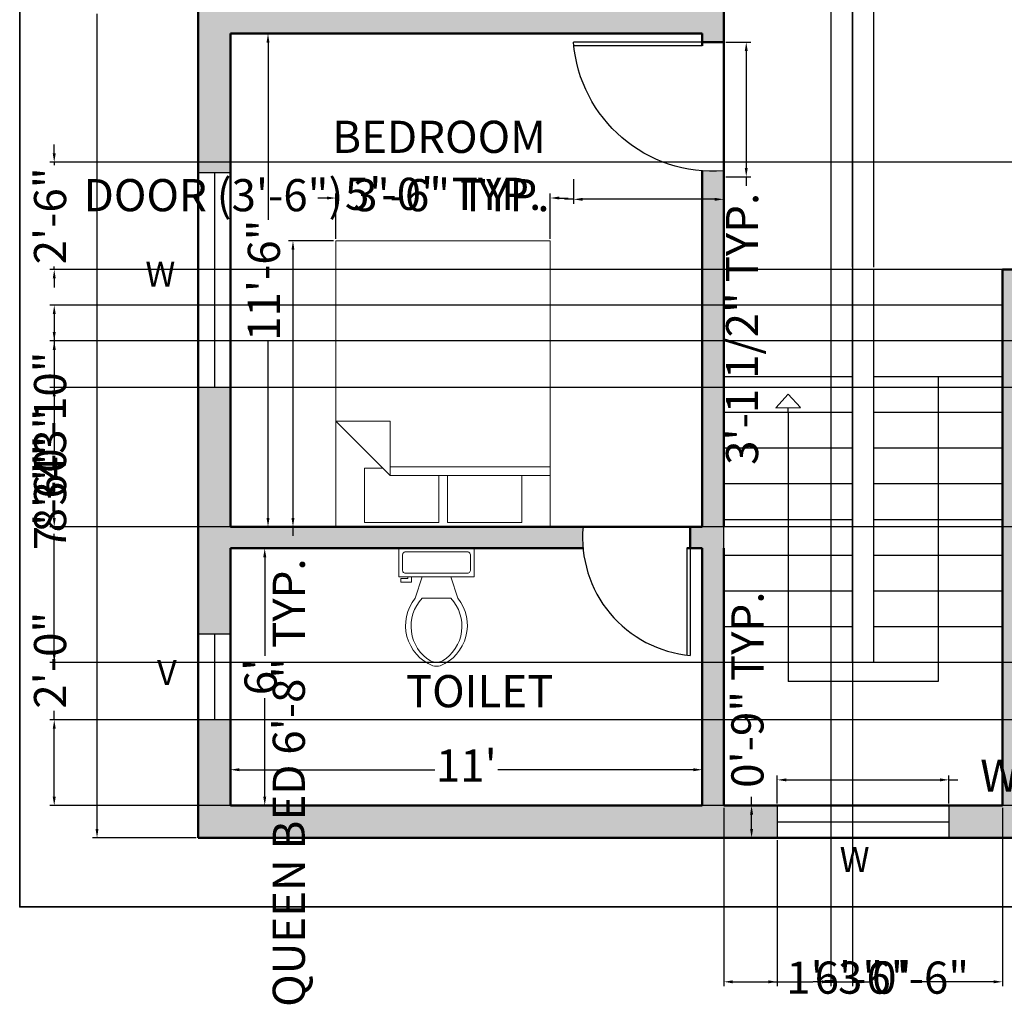
# Model space of a CAD drawing. Units: inches. Extents: x 2463 to 3327, y 6994 to 7582.
# Tile 1 of 5: x 2463 to 2739, y 6994 to 7270. Entities that reach past the tile are written whole.
import ezdxf

# ---------------------------------------------------------------- set-up
doc = ezdxf.new("R2010")
doc.units = ezdxf.units.IN
for name, color, linetype, lineweight in [('A-ANNO-DIMS', 2, 'Continuous', 18), ('A-ANNO-TEXT', 7, 'Continuous', 18), ('A-ANNO-TTLB', 7, 'Continuous', 35), ('A-AREA-IDEN', 3, 'Continuous', 25), ('A-DOOR', 4, 'Continuous', 25), ('A-FLOR-FIXT', 8, 'Continuous', 18), ('A-FLOR-STRS', 3, 'Continuous', 25), ('A-FURN', 8, 'Continuous', 18), ('A-GLAZ', 4, 'Continuous', 25), ('A-WALL', 7, 'Continuous', 50), ('A-WALL-PATT', 252, 'Continuous', 13)]:
    doc.layers.add(name, color=color, linetype=linetype, lineweight=lineweight)
doc.styles.get("Standard").update_dxf_attribs({"font": 'times.ttf'})
doc.dimstyles.new('ISO-25', dxfattribs={"dimtxt": 9, "dimasz": 2.5, "dimexe": 1.25, "dimexo": 0.625, "dimgap": 2, "dimtad": 0, "dimdec": 1, "dimlunit": 4, "dimtxsty": 'Standard', "dimcen": 2.5, "dimadec": 0, "dimazin": 0, "dimtfac": 1, "dimtdec": 1, "dimtmove": 0, "dimatfit": 3, "dimfxl": 1, "dimarcsym": 0})

# ---------------------------------------------------------------- blocks, each defined once
blk = doc.blocks.new('*D6')
at = {"layer": 'A-ANNO-DIMS', "color": 0, "lineweight": -2, "transparency": 16777216}
for p, q in [((2522.43, 7050.45), (2522.43, 7061.12)), ((2654.43, 7050.45), (2654.43, 7061.12)), ((2524.93, 7059.87), (2579.65, 7059.87)), ((2651.93, 7059.87), (2597.21, 7059.87))]:
    blk.add_line(p, q, dxfattribs=at)
at = {"layer": 'A-ANNO-DIMS', "color": 0, "transparency": 16777216}
for points in [[(2524.93, 7060.29), (2524.93, 7059.45), (2522.43, 7059.87)], [(2651.93, 7060.29), (2651.93, 7059.45), (2654.43, 7059.87)]]:
    blk.add_solid(points, dxfattribs=at)
at = {"layer": 'Defpoints', "color": 0, "transparency": 16777216}
for p in [(2654.43, 7059.87), (2522.43, 7049.83), (2654.43, 7049.83)]:
    blk.add_point(p, dxfattribs=at)
at = {"layer": 'A-ANNO-DIMS', "color": 0, "transparency": 16777216, "insert": (2588.43, 7059.87), "char_height": 9, "attachment_point": 5}
blk.add_mtext("11'", dxfattribs=at)
blk = doc.blocks.new('*D7')
at = {"layer": 'A-ANNO-DIMS', "color": 0, "lineweight": -2, "transparency": 16777216}
for p, q in [((2523.06, 7121.83), (2533.27, 7121.83)), ((2532.02, 7119.33), (2532.02, 7091.78)), ((2532.02, 7052.33), (2532.02, 7079.87)), ((2523.06, 7049.83), (2533.27, 7049.83))]:
    blk.add_line(p, q, dxfattribs=at)
at = {"layer": 'A-ANNO-DIMS', "color": 0, "transparency": 16777216}
for points in [[(2531.61, 7119.33), (2532.44, 7119.33), (2532.02, 7121.83)], [(2531.61, 7052.33), (2532.44, 7052.33), (2532.02, 7049.83)]]:
    blk.add_solid(points, dxfattribs=at)
at = {"layer": 'Defpoints', "color": 0, "transparency": 16777216}
for p in [(2522.43, 7121.83), (2532.02, 7121.83), (2522.43, 7049.83)]:
    blk.add_point(p, dxfattribs=at)
at = {"layer": 'A-ANNO-DIMS', "color": 0, "transparency": 16777216, "insert": (2532.02, 7085.83), "char_height": 9, "attachment_point": 5, "rotation": 90}
blk.add_mtext("6'", dxfattribs=at)
blk = doc.blocks.new('*D8')
at = {"layer": 'A-ANNO-DIMS', "color": 0, "lineweight": -2, "transparency": 16777216}
for p, q in [((2523.06, 7265.83), (2534.19, 7265.83)), ((2532.94, 7263.33), (2532.94, 7213.69)), ((2532.94, 7130.33), (2532.94, 7179.96)), ((2523.06, 7127.83), (2534.19, 7127.83))]:
    blk.add_line(p, q, dxfattribs=at)
at = {"layer": 'A-ANNO-DIMS', "color": 0, "transparency": 16777216}
for points in [[(2532.52, 7263.33), (2533.35, 7263.33), (2532.94, 7265.83)], [(2532.52, 7130.33), (2533.35, 7130.33), (2532.94, 7127.83)]]:
    blk.add_solid(points, dxfattribs=at)
at = {"layer": 'Defpoints', "color": 0, "transparency": 16777216}
for p in [(2522.43, 7265.83), (2532.94, 7265.83), (2522.43, 7127.83)]:
    blk.add_point(p, dxfattribs=at)
at = {"layer": 'A-ANNO-DIMS', "color": 0, "transparency": 16777216, "insert": (2532.94, 7196.83), "char_height": 9, "attachment_point": 5, "rotation": 90}
blk.add_mtext('11\'-6"', dxfattribs=at)
blk = doc.blocks.new('Bed - Queen')
for p, q in [((0, -80.00003), (0, 0)), ((0, 0), (59.99999, 0)), ((59.99999, 0), (59.99999, -80.00003)), ((7.99999, -1.2), (28.79998, -1.2)), ((7.99999, -14.4), (7.99999, -1.2)), ((28.79998, -1.2), (28.79998, -14.4)), ((31.19999, -1.2), (51.99999, -1.2)), ((31.19999, -14.4), (31.19999, -1.2)), ((51.99999, -1.2), (51.99999, -16.4)), ((0, -14.4), (44.8, -14.4)), ((59.99999, -29.6), (44.8, -14.4)), ((44.8, -14.4), (44.8, -29.6)), ((51.99999, -16.4), (46.79936, -16.4)), ((44.8, -16.8), (0, -16.8)), ((44.8, -29.6), (59.99999, -29.6)), ((59.99999, -80.00003), (0, -80.00003))]:
    blk.add_line(p, q)
blk = doc.blocks.new('*U11')
for p, q in [((9.5, -6), (9.5, -2)), ((-8, -8.5), (-8, -8)), ((-7, -8), (-7, -9.5)), ((-4, -8), (-6, -14)), ((4, -8), (6, -14)), ((-10, -8.5), (-8, -8.5)), ((-10, -9.5), (-10, -8.5)), ((-7, -9.5), (-10, -9.5)), ((4, -14), (-4, -14))]:
    blk.add_line(p, q)
blk.add_lwpolyline([(10.5, -8), (10.5, 0), (-10.5, 0), (-10.5, -8)], close=True)
for points in [[(-9.5, -2), (-9.5, -6)], [(8.5, -1), (-8.5, -1)], [(-8.5, -7), (8.5, -7)]]:
    blk.add_lwpolyline(points)
for centre, radius, start, end in [((-8.62, -1.88), 0.884, 81.8699, 188.1301), ((8.62, -1.88), 0.884, 351.8699, 98.1301), ((-8.62, -6.12), 0.884, 171.8699, 278.1301), ((8.62, -6.12), 0.884, 261.8699, 8.1301), ((3.52, -21.58), 12.17, 141.4691, 247.9714), ((4.2, -21.82), 11.33, 136.3677, 238.9468), ((-3.52, -21.58), 12.17, 292.0284, 38.5307), ((-4.2, -21.82), 11.33, 301.053, 43.6321), ((0, -27.88), 4, 245.7318, 294.2682), ((0, -29), 4, 254.8605, 285.1395)]:
    blk.add_arc(centre, radius, start, end)
blk = doc.blocks.new('*D26')
at = {"layer": 'A-ANNO-DIMS', "color": 0, "lineweight": -2, "transparency": 16777216}
for p, q in [((2512.81, 7520.83), (2483.85, 7520.83)), ((2485.1, 7518.33), (2485.1, 7290.28)), ((2485.1, 7043.33), (2485.1, 7271.37)), ((2512.81, 7040.83), (2483.85, 7040.83))]:
    blk.add_line(p, q, dxfattribs=at)
at = {"layer": 'A-ANNO-DIMS', "color": 0, "transparency": 16777216}
for points in [[(2484.68, 7518.33), (2485.51, 7518.33), (2485.1, 7520.83)], [(2484.68, 7043.33), (2485.51, 7043.33), (2485.1, 7040.83)]]:
    blk.add_solid(points, dxfattribs=at)
at = {"layer": 'Defpoints', "color": 0, "transparency": 16777216}
for p in [(2513.43, 7520.83), (2485.1, 7040.83), (2513.43, 7040.83)]:
    blk.add_point(p, dxfattribs=at)
at = {"layer": 'A-ANNO-DIMS', "color": 0, "transparency": 16777216, "insert": (2485.1, 7280.83), "char_height": 9, "attachment_point": 5, "rotation": 90}
blk.add_mtext("40'", dxfattribs=at)
blk = doc.blocks.new('DOOR-36')
for p, q in [((0, 6), (0, 42)), ((1, 6), (1, 41.91))]:
    blk.add_line(p, q)
blk.add_arc((-3, 3), 39.12, 355.6013, 85.6013)
blk = doc.blocks.new('DOOR-30')
for p, q in [((29.14, 30), (29.14, 0)), ((30.14, 30), (30.14, 0))]:
    blk.add_line(p, q)
blk.add_arc((33.14, 33), 33.14, 174.8056, 264.8056)
blk = doc.blocks.new('WIN-60')
for p, q in [((9, 60), (0, 60)), ((4.5, 60), (4.5, 0)), ((9, 0), (0, 0))]:
    blk.add_line(p, q)
blk = doc.blocks.new('WIN-24')
for p, q in [((9, 24), (0, 24)), ((4.5, 24), (4.5, 0)), ((9, 0), (0, 0))]:
    blk.add_line(p, q)
blk = doc.blocks.new('WIN-48')
for p, q in [((0, 9), (0, 0)), ((48, 9), (48, 0)), ((0, 4.5), (48, 4.5))]:
    blk.add_line(p, q)
blk = doc.blocks.new('*D33')
at = {"layer": 'A-ANNO-DIMS', "color": 0, "lineweight": -2, "transparency": 16777216}
for p, q in [((2551.29, 7207.83), (2538.67, 7207.83)), ((2539.92, 7205.33), (2539.92, 7130.33)), ((2551.29, 7127.83), (2538.67, 7127.83)), ((2539.92, 7127.83), (2539.92, 7125.33))]:
    blk.add_line(p, q, dxfattribs=at)
at = {"layer": 'A-ANNO-DIMS', "color": 0, "transparency": 16777216}
for points in [[(2539.5, 7205.33), (2540.33, 7205.33), (2539.92, 7207.83)], [(2539.5, 7130.33), (2540.33, 7130.33), (2539.92, 7127.83)]]:
    blk.add_solid(points, dxfattribs=at)
at = {"layer": 'Defpoints', "color": 0, "transparency": 16777216}
for p in [(2551.92, 7207.83), (2539.92, 7127.83), (2551.92, 7127.83)]:
    blk.add_point(p, dxfattribs=at)
at = {"layer": 'A-ANNO-DIMS', "color": 0, "transparency": 16777216, "insert": (2539.92, 7056.26), "char_height": 9, "attachment_point": 5, "rotation": 90}
blk.add_mtext('QUEEN BED 6\'-8" TYP.', dxfattribs=at)
blk = doc.blocks.new('*D34')
at = {"layer": 'A-ANNO-DIMS', "color": 0, "lineweight": -2, "transparency": 16777216}
for p, q in [((2551.92, 7208.45), (2551.92, 7221.08)), ((2611.92, 7208.45), (2611.92, 7221.08)), ((2549.42, 7219.83), (2546.92, 7219.83)), ((2551.92, 7219.83), (2552.06, 7219.83)), ((2611.92, 7219.83), (2611.77, 7219.83)), ((2614.42, 7219.83), (2616.92, 7219.83))]:
    blk.add_line(p, q, dxfattribs=at)
at = {"layer": 'A-ANNO-DIMS', "color": 0, "transparency": 16777216}
for points in [[(2549.42, 7220.24), (2549.42, 7219.41), (2551.92, 7219.83)], [(2614.42, 7220.24), (2614.42, 7219.41), (2611.92, 7219.83)]]:
    blk.add_solid(points, dxfattribs=at)
at = {"layer": 'Defpoints', "color": 0, "transparency": 16777216}
for p in [(2551.92, 7219.83), (2551.92, 7207.83), (2611.92, 7207.83)]:
    blk.add_point(p, dxfattribs=at)
at = {"layer": 'A-ANNO-DIMS', "color": 0, "transparency": 16777216, "insert": (2581.92, 7219.83), "char_height": 9, "attachment_point": 5}
blk.add_mtext('5\'-0" TYP.', dxfattribs=at)
blk = doc.blocks.new('*D41')
at = {"layer": 'A-ANNO-DIMS', "color": 0, "lineweight": -2, "transparency": 16777216}
for p, q in [((2675.43, 7050.45), (2675.43, 7058.28)), ((2723.43, 7050.45), (2723.43, 7058.28)), ((2677.93, 7057.03), (2720.93, 7057.03)), ((2723.43, 7057.03), (2725.93, 7057.03))]:
    blk.add_line(p, q, dxfattribs=at)
at = {"layer": 'A-ANNO-DIMS', "color": 0, "transparency": 16777216}
for points in [[(2677.93, 7057.44), (2677.93, 7056.61), (2675.43, 7057.03)], [(2720.93, 7057.44), (2720.93, 7056.61), (2723.43, 7057.03)]]:
    blk.add_solid(points, dxfattribs=at)
at = {"layer": 'Defpoints', "color": 0, "transparency": 16777216}
for p in [(2723.43, 7057.03), (2675.43, 7049.83), (2723.43, 7049.83)]:
    blk.add_point(p, dxfattribs=at)
at = {"layer": 'A-ANNO-DIMS', "color": 0, "transparency": 16777216, "insert": (2786.83, 7057.03), "char_height": 9, "attachment_point": 5}
blk.add_mtext('WINDOW 4\'-0" TYP.', dxfattribs=at)
blk = doc.blocks.new('*D42')
at = {"layer": 'A-ANNO-DIMS', "color": 0, "lineweight": -2, "transparency": 16777216}
for p, q in [((2674.81, 7049.83), (2666.98, 7049.83)), ((2668.23, 7049.83), (2668.23, 7052.33)), ((2668.23, 7043.33), (2668.23, 7047.33)), ((2674.81, 7040.83), (2666.98, 7040.83))]:
    blk.add_line(p, q, dxfattribs=at)
at = {"layer": 'A-ANNO-DIMS', "color": 0, "transparency": 16777216}
for points in [[(2667.81, 7047.33), (2668.65, 7047.33), (2668.23, 7049.83)], [(2667.81, 7043.33), (2668.65, 7043.33), (2668.23, 7040.83)]]:
    blk.add_solid(points, dxfattribs=at)
at = {"layer": 'Defpoints', "color": 0, "transparency": 16777216}
for p in [(2668.23, 7049.83), (2675.43, 7049.83), (2675.43, 7040.83)]:
    blk.add_point(p, dxfattribs=at)
at = {"layer": 'A-ANNO-DIMS', "color": 0, "transparency": 16777216, "insert": (2668.23, 7082.26), "char_height": 9, "attachment_point": 5, "rotation": 90}
blk.add_mtext('0\'-9" TYP.', dxfattribs=at)
blk = doc.blocks.new('*D45')
at = {"layer": 'A-ANNO-DIMS', "color": 0, "lineweight": -2, "transparency": 16777216}
for p, q in [((2618.43, 7225.14), (2618.43, 7218.21)), ((2660.43, 7225.14), (2660.43, 7218.21)), ((2618.43, 7219.46), (2615.93, 7219.46)), ((2657.93, 7219.46), (2620.93, 7219.46))]:
    blk.add_line(p, q, dxfattribs=at)
at = {"layer": 'A-ANNO-DIMS', "color": 0, "transparency": 16777216}
for points in [[(2620.93, 7219.88), (2620.93, 7219.04), (2618.43, 7219.46)], [(2657.93, 7219.88), (2657.93, 7219.04), (2660.43, 7219.46)]]:
    blk.add_solid(points, dxfattribs=at)
at = {"layer": 'Defpoints', "color": 0, "transparency": 16777216}
for p in [(2618.43, 7225.76), (2660.43, 7225.76), (2618.43, 7219.46)]:
    blk.add_point(p, dxfattribs=at)
at = {"layer": 'A-ANNO-DIMS', "color": 0, "transparency": 16777216, "insert": (2546.53, 7219.46), "char_height": 9, "attachment_point": 5}
blk.add_mtext('DOOR (3\'-6") 3\'-6" TYP.', dxfattribs=at)
blk = doc.blocks.new('*D46')
at = {"layer": 'A-ANNO-DIMS', "color": 0, "lineweight": -2, "transparency": 16777216}
for p, q in [((2661.06, 7263.42), (2667.98, 7263.42)), ((2666.73, 7260.92), (2666.73, 7228.26)), ((2661.06, 7225.76), (2667.98, 7225.76)), ((2666.73, 7225.76), (2666.73, 7223.26))]:
    blk.add_line(p, q, dxfattribs=at)
at = {"layer": 'A-ANNO-DIMS', "color": 0, "transparency": 16777216}
for points in [[(2666.31, 7260.92), (2667.15, 7260.92), (2666.73, 7263.42)], [(2666.31, 7228.26), (2667.15, 7228.26), (2666.73, 7225.76)]]:
    blk.add_solid(points, dxfattribs=at)
at = {"layer": 'Defpoints', "color": 0, "transparency": 16777216}
for p in [(2660.43, 7263.42), (2660.43, 7225.76), (2666.73, 7225.76)]:
    blk.add_point(p, dxfattribs=at)
at = {"layer": 'A-ANNO-DIMS', "color": 0, "transparency": 16777216, "insert": (2666.73, 7183.21), "char_height": 9, "attachment_point": 5, "rotation": 90}
blk.add_mtext('3\'-1 1/2" TYP.', dxfattribs=at)
blk = doc.blocks.new('*D49')
at = {"layer": 'A-ANNO-DIMS', "color": 0, "lineweight": -2, "transparency": 16777216}
for p, q in [((2696.43, 7391.2), (2696.43, 6999.28)), ((2690.43, 7385.2), (2690.43, 6999.28)), ((2687.93, 7000.53), (2685.43, 7000.53)), ((2690.43, 7000.53), (2696.43, 7000.53)), ((2698.93, 7000.53), (2701.43, 7000.53))]:
    blk.add_line(p, q, dxfattribs=at)
at = {"layer": 'A-ANNO-DIMS', "color": 0, "transparency": 16777216}
for points in [[(2687.93, 7000.94), (2687.93, 7000.11), (2690.43, 7000.53)], [(2698.93, 7000.94), (2698.93, 7000.11), (2696.43, 7000.53)]]:
    blk.add_solid(points, dxfattribs=at)
at = {"layer": 'Defpoints', "color": 0, "transparency": 16777216}
for p in [(2696.43, 7391.83), (2690.43, 7385.83), (2696.43, 7000.53)]:
    blk.add_point(p, dxfattribs=at)
at = {"layer": 'A-ANNO-DIMS', "color": 0, "transparency": 16777216, "insert": (2715.52, 7000.53), "char_height": 9, "attachment_point": 5}
blk.add_mtext('0\'-6"', dxfattribs=at)
blk = doc.blocks.new('*D52')
at = {"layer": 'A-ANNO-DIMS', "color": 0, "lineweight": -2, "transparency": 16777216}
for p, q in [((2660.43, 7272.45), (2660.43, 7562.38)), ((2786.43, 7230.45), (2786.43, 7562.38)), ((2662.93, 7561.13), (2706.56, 7561.13)), ((2783.93, 7561.13), (2740.3, 7561.13))]:
    blk.add_line(p, q, dxfattribs=at)
at = {"layer": 'A-ANNO-DIMS', "color": 0, "transparency": 16777216}
for points in [[(2662.93, 7561.54), (2662.93, 7560.71), (2660.43, 7561.13)], [(2783.93, 7561.54), (2783.93, 7560.71), (2786.43, 7561.13)]]:
    blk.add_solid(points, dxfattribs=at)
at = {"layer": 'Defpoints', "color": 0, "transparency": 16777216}
for p in [(2786.43, 7561.13), (2660.43, 7271.83), (2786.43, 7229.83)]:
    blk.add_point(p, dxfattribs=at)
at = {"layer": 'A-ANNO-DIMS', "color": 0, "transparency": 16777216, "insert": (2723.43, 7561.13), "char_height": 9, "attachment_point": 5}
blk.add_mtext('10\'-6"', dxfattribs=at)
blk = doc.blocks.new('*D53')
at = {"layer": 'A-ANNO-DIMS', "color": 0, "lineweight": -2, "transparency": 16777216}
for p, q in [((2473.13, 7232.33), (2473.13, 7234.83)), ((2785.81, 7229.83), (2471.88, 7229.83)), ((2473.13, 7229.83), (2473.13, 7229.01)), ((2737.81, 7199.83), (2471.88, 7199.83)), ((2473.13, 7199.83), (2473.13, 7200.64)), ((2473.13, 7197.33), (2473.13, 7194.83))]:
    blk.add_line(p, q, dxfattribs=at)
at = {"layer": 'A-ANNO-DIMS', "color": 0, "transparency": 16777216}
for points in [[(2472.71, 7232.33), (2473.55, 7232.33), (2473.13, 7229.83)], [(2472.71, 7197.33), (2473.55, 7197.33), (2473.13, 7199.83)]]:
    blk.add_solid(points, dxfattribs=at)
at = {"layer": 'Defpoints', "color": 0, "transparency": 16777216}
for p in [(2473.13, 7229.83), (2786.43, 7229.83), (2738.43, 7199.83)]:
    blk.add_point(p, dxfattribs=at)
at = {"layer": 'A-ANNO-DIMS', "color": 0, "transparency": 16777216, "insert": (2473.13, 7214.83), "char_height": 9, "attachment_point": 5, "rotation": 90}
blk.add_mtext('2\'-6"', dxfattribs=at)
blk = doc.blocks.new('*D54')
at = {"layer": 'A-ANNO-DIMS', "color": 0, "lineweight": -2, "transparency": 16777216}
for p, q in [((2660.43, 7049.2), (2660.43, 6999.28)), ((2738.43, 7049.2), (2738.43, 6999.28)), ((2662.93, 7000.53), (2685.39, 7000.53)), ((2735.93, 7000.53), (2713.47, 7000.53))]:
    blk.add_line(p, q, dxfattribs=at)
at = {"layer": 'A-ANNO-DIMS', "color": 0, "transparency": 16777216}
for points in [[(2662.93, 7000.94), (2662.93, 7000.11), (2660.43, 7000.53)], [(2735.93, 7000.94), (2735.93, 7000.11), (2738.43, 7000.53)]]:
    blk.add_solid(points, dxfattribs=at)
at = {"layer": 'Defpoints', "color": 0, "transparency": 16777216}
for p in [(2660.43, 7049.83), (2738.43, 7049.83), (2738.43, 7000.53)]:
    blk.add_point(p, dxfattribs=at)
at = {"layer": 'A-ANNO-DIMS', "color": 0, "transparency": 16777216, "insert": (2699.43, 7000.53), "char_height": 9, "attachment_point": 5}
blk.add_mtext('6\'-6"', dxfattribs=at)
blk = doc.blocks.new('*D55')
at = {"layer": 'A-ANNO-DIMS', "color": 0, "lineweight": -2, "transparency": 16777216}
for p, q in [((2660.43, 7190.45), (2660.43, 7562.38)), ((2696.43, 7200.45), (2696.43, 7562.38)), ((2657.93, 7561.13), (2655.43, 7561.13)), ((2660.43, 7561.13), (2664.38, 7561.13)), ((2696.43, 7561.13), (2692.49, 7561.13)), ((2698.93, 7561.13), (2701.43, 7561.13))]:
    blk.add_line(p, q, dxfattribs=at)
at = {"layer": 'A-ANNO-DIMS', "color": 0, "transparency": 16777216}
for points in [[(2657.93, 7561.54), (2657.93, 7560.71), (2660.43, 7561.13)], [(2698.93, 7561.54), (2698.93, 7560.71), (2696.43, 7561.13)]]:
    blk.add_solid(points, dxfattribs=at)
at = {"layer": 'Defpoints', "color": 0, "transparency": 16777216}
for p in [(2696.43, 7561.13), (2696.43, 7199.83), (2660.43, 7189.83)]:
    blk.add_point(p, dxfattribs=at)
at = {"layer": 'A-ANNO-DIMS', "color": 0, "transparency": 16777216, "insert": (2678.43, 7561.13), "char_height": 9, "attachment_point": 5}
blk.add_mtext('3\'-0"', dxfattribs=at)
blk = doc.blocks.new('*D56')
at = {"layer": 'A-ANNO-DIMS', "color": 0, "lineweight": -2, "transparency": 16777216}
for p, q in [((2696.43, 7200.45), (2696.43, 7562.38)), ((2702.43, 7200.45), (2702.43, 7562.38)), ((2693.93, 7561.13), (2691.43, 7561.13)), ((2696.43, 7561.13), (2702.43, 7561.13)), ((2704.93, 7561.13), (2707.43, 7561.13))]:
    blk.add_line(p, q, dxfattribs=at)
at = {"layer": 'A-ANNO-DIMS', "color": 0, "transparency": 16777216}
for points in [[(2693.93, 7561.54), (2693.93, 7560.71), (2696.43, 7561.13)], [(2704.93, 7561.54), (2704.93, 7560.71), (2702.43, 7561.13)]]:
    blk.add_solid(points, dxfattribs=at)
at = {"layer": 'Defpoints', "color": 0, "transparency": 16777216}
for p in [(2702.43, 7561.13), (2696.43, 7199.83), (2702.43, 7199.83)]:
    blk.add_point(p, dxfattribs=at)
at = {"layer": 'A-ANNO-DIMS', "color": 0, "transparency": 16777216, "insert": (2721.52, 7561.13), "char_height": 9, "attachment_point": 5}
blk.add_mtext('0\'-6"', dxfattribs=at)
blk = doc.blocks.new('*D57')
at = {"layer": 'A-ANNO-DIMS', "color": 0, "lineweight": -2, "transparency": 16777216}
for p, q in [((2737.81, 7189.83), (2471.88, 7189.83)), ((2473.13, 7187.33), (2473.13, 7182.33)), ((2737.81, 7179.83), (2471.88, 7179.83)), ((2473.13, 7179.83), (2473.13, 7177.33))]:
    blk.add_line(p, q, dxfattribs=at)
at = {"layer": 'A-ANNO-DIMS', "color": 0, "transparency": 16777216}
for points in [[(2472.71, 7187.33), (2473.55, 7187.33), (2473.13, 7189.83)], [(2472.71, 7182.33), (2473.55, 7182.33), (2473.13, 7179.83)]]:
    blk.add_solid(points, dxfattribs=at)
at = {"layer": 'Defpoints', "color": 0, "transparency": 16777216}
for p in [(2738.43, 7189.83), (2473.13, 7179.83), (2738.43, 7179.83)]:
    blk.add_point(p, dxfattribs=at)
at = {"layer": 'A-ANNO-DIMS', "color": 0, "transparency": 16777216, "insert": (2473.13, 7159.92), "char_height": 9, "attachment_point": 5, "rotation": 90}
blk.add_mtext('0\'-10"', dxfattribs=at)
blk = doc.blocks.new('*D58')
at = {"layer": 'A-ANNO-DIMS', "color": 0, "lineweight": -2, "transparency": 16777216}
for p, q in [((2659.81, 7189.83), (2471.88, 7189.83)), ((2473.13, 7187.33), (2473.13, 7153.75)), ((2473.13, 7092.33), (2473.13, 7125.9)), ((2659.81, 7089.83), (2471.88, 7089.83))]:
    blk.add_line(p, q, dxfattribs=at)
at = {"layer": 'A-ANNO-DIMS', "color": 0, "transparency": 16777216}
for points in [[(2472.71, 7187.33), (2473.55, 7187.33), (2473.13, 7189.83)], [(2472.71, 7092.33), (2473.55, 7092.33), (2473.13, 7089.83)]]:
    blk.add_solid(points, dxfattribs=at)
at = {"layer": 'Defpoints', "color": 0, "transparency": 16777216}
for p in [(2660.43, 7189.83), (2473.13, 7089.83), (2660.43, 7089.83)]:
    blk.add_point(p, dxfattribs=at)
at = {"layer": 'A-ANNO-DIMS', "color": 0, "transparency": 16777216, "insert": (2473.13, 7139.83), "char_height": 9, "attachment_point": 5, "rotation": 90}
blk.add_mtext('8\'-4"', dxfattribs=at)
blk = doc.blocks.new('*D60')
at = {"layer": 'A-ANNO-DIMS', "color": 0, "lineweight": -2, "transparency": 16777216}
for p, q in [((2473.13, 7073.83), (2473.13, 7076.33)), ((2521.81, 7073.83), (2471.88, 7073.83)), ((2473.13, 7052.33), (2473.13, 7071.33)), ((2521.81, 7049.83), (2471.88, 7049.83))]:
    blk.add_line(p, q, dxfattribs=at)
at = {"layer": 'A-ANNO-DIMS', "color": 0, "transparency": 16777216}
for points in [[(2472.71, 7071.33), (2473.55, 7071.33), (2473.13, 7073.83)], [(2472.71, 7052.33), (2473.55, 7052.33), (2473.13, 7049.83)]]:
    blk.add_solid(points, dxfattribs=at)
at = {"layer": 'Defpoints', "color": 0, "transparency": 16777216}
for p in [(2473.13, 7073.83), (2522.43, 7073.83), (2522.43, 7049.83)]:
    blk.add_point(p, dxfattribs=at)
at = {"layer": 'A-ANNO-DIMS', "color": 0, "transparency": 16777216, "insert": (2473.13, 7090.51), "char_height": 9, "attachment_point": 5, "rotation": 90}
blk.add_mtext('2\'-0"', dxfattribs=at)
blk = doc.blocks.new('*D61')
at = {"layer": 'A-ANNO-DIMS', "color": 0, "lineweight": -2, "transparency": 16777216}
for p, q in [((2521.81, 7166.83), (2471.88, 7166.83)), ((2473.13, 7164.33), (2473.13, 7161.38)), ((2473.13, 7130.33), (2473.13, 7133.27)), ((2521.81, 7127.83), (2471.88, 7127.83))]:
    blk.add_line(p, q, dxfattribs=at)
at = {"layer": 'A-ANNO-DIMS', "color": 0, "transparency": 16777216}
for points in [[(2472.71, 7164.33), (2473.55, 7164.33), (2473.13, 7166.83)], [(2472.71, 7130.33), (2473.55, 7130.33), (2473.13, 7127.83)]]:
    blk.add_solid(points, dxfattribs=at)
at = {"layer": 'Defpoints', "color": 0, "transparency": 16777216}
for p in [(2473.13, 7166.83), (2522.43, 7166.83), (2522.43, 7127.83)]:
    blk.add_point(p, dxfattribs=at)
at = {"layer": 'A-ANNO-DIMS', "color": 0, "transparency": 16777216, "insert": (2473.13, 7147.33), "char_height": 9, "attachment_point": 5, "rotation": 90}
blk.add_mtext('3\'-3"', dxfattribs=at)
blk = doc.blocks.new('*D66')
at = {"layer": 'A-ANNO-DIMS', "color": 0, "lineweight": -2, "transparency": 16777216}
for p, q in [((2660.43, 7049.2), (2660.43, 6999.28)), ((2675.43, 7040.2), (2675.43, 6999.28)), ((2662.93, 7000.53), (2672.93, 7000.53)), ((2675.43, 7000.53), (2677.93, 7000.53))]:
    blk.add_line(p, q, dxfattribs=at)
at = {"layer": 'A-ANNO-DIMS', "color": 0, "transparency": 16777216}
for points in [[(2662.93, 7000.94), (2662.93, 7000.11), (2660.43, 7000.53)], [(2672.93, 7000.94), (2672.93, 7000.11), (2675.43, 7000.53)]]:
    blk.add_solid(points, dxfattribs=at)
at = {"layer": 'Defpoints', "color": 0, "transparency": 16777216}
for p in [(2660.43, 7049.83), (2675.43, 7040.83), (2675.43, 7000.53)]:
    blk.add_point(p, dxfattribs=at)
at = {"layer": 'A-ANNO-DIMS', "color": 0, "transparency": 16777216, "insert": (2691.48, 7000.53), "char_height": 9, "attachment_point": 5}
blk.add_mtext('1\'-3"', dxfattribs=at)
blk = doc.blocks.new('*D75')
at = {"layer": 'A-ANNO-DIMS', "color": 0, "lineweight": -2, "transparency": 16777216}
for p, q in [((3144.8, 7179.83), (2471.88, 7179.83)), ((2473.13, 7177.33), (2473.13, 7148.9)), ((2473.13, 7092.33), (2473.13, 7120.75)), ((3144.8, 7089.83), (2471.88, 7089.83))]:
    blk.add_line(p, q, dxfattribs=at)
at = {"layer": 'A-ANNO-DIMS', "color": 0, "transparency": 16777216}
for points in [[(2472.71, 7177.33), (2473.55, 7177.33), (2473.13, 7179.83)], [(2472.71, 7092.33), (2473.55, 7092.33), (2473.13, 7089.83)]]:
    blk.add_solid(points, dxfattribs=at)
at = {"layer": 'Defpoints', "color": 0, "transparency": 16777216}
for p in [(3145.42, 7179.83), (2473.13, 7089.83), (3145.42, 7089.83)]:
    blk.add_point(p, dxfattribs=at)
at = {"layer": 'A-ANNO-DIMS', "color": 0, "transparency": 16777216, "insert": (2473.13, 7134.83), "char_height": 9, "attachment_point": 5, "rotation": 90}
blk.add_mtext('7\'-6"', dxfattribs=at)
blk = doc.blocks.new('*D76')
at = {"layer": 'A-ANNO-DIMS', "color": 0, "lineweight": -2, "transparency": 16777216}
for p, q in [((2473.13, 7073.83), (2473.13, 7076.33)), ((2928.8, 7073.83), (2471.88, 7073.83)), ((2473.13, 7052.33), (2473.13, 7071.33)), ((2928.8, 7049.83), (2471.88, 7049.83))]:
    blk.add_line(p, q, dxfattribs=at)
at = {"layer": 'A-ANNO-DIMS', "color": 0, "transparency": 16777216}
for points in [[(2472.71, 7071.33), (2473.55, 7071.33), (2473.13, 7073.83)], [(2472.71, 7052.33), (2473.55, 7052.33), (2473.13, 7049.83)]]:
    blk.add_solid(points, dxfattribs=at)
at = {"layer": 'Defpoints', "color": 0, "transparency": 16777216}
for p in [(2473.13, 7073.83), (2929.42, 7073.83), (2929.42, 7049.83)]:
    blk.add_point(p, dxfattribs=at)
at = {"layer": 'A-ANNO-DIMS', "color": 0, "transparency": 16777216, "insert": (2473.13, 7090.51), "char_height": 9, "attachment_point": 5, "rotation": 90}
blk.add_mtext('2\'-0"', dxfattribs=at)
blk = doc.blocks.new('*D77')
at = {"layer": 'A-ANNO-DIMS', "color": 0, "lineweight": -2, "transparency": 16777216}
for p, q in [((2928.8, 7166.83), (2471.88, 7166.83)), ((2473.13, 7164.33), (2473.13, 7161.38)), ((2473.13, 7130.33), (2473.13, 7133.27)), ((2928.8, 7127.83), (2471.88, 7127.83))]:
    blk.add_line(p, q, dxfattribs=at)
at = {"layer": 'A-ANNO-DIMS', "color": 0, "transparency": 16777216}
for points in [[(2472.71, 7164.33), (2473.55, 7164.33), (2473.13, 7166.83)], [(2472.71, 7130.33), (2473.55, 7130.33), (2473.13, 7127.83)]]:
    blk.add_solid(points, dxfattribs=at)
at = {"layer": 'Defpoints', "color": 0, "transparency": 16777216}
for p in [(2473.13, 7166.83), (2929.42, 7166.83), (2929.42, 7127.83)]:
    blk.add_point(p, dxfattribs=at)
at = {"layer": 'A-ANNO-DIMS', "color": 0, "transparency": 16777216, "insert": (2473.13, 7147.33), "char_height": 9, "attachment_point": 5, "rotation": 90}
blk.add_mtext('3\'-3"', dxfattribs=at)

msp = doc.modelspace()

# ---------------------------------------------------------------- hatches: boundary and pattern name
at = {"layer": 'A-WALL-PATT'}
h = msp.add_hatch(color=256, dxfattribs=at)
h.dxf.hatch_style = 1
h.paths.add_polyline_path([(2522.43, 7511.83), (2690.43, 7511.83), (2690.43, 7385.83), (2696.43, 7385.83), (2702.68, 7385.83), (2702.68, 7391.83), (2696.43, 7391.83), (2696.43, 7511.83), (2864.43, 7511.83), (2864.43, 7481.83), (2873.43, 7481.83), (2873.43, 7520.83), (2513.43, 7520.83), (2513.43, 7501.71), (2522.43, 7501.71)])
h.paths.add_polyline_path([(2522.43, 7453.71, -0.042779), (2513.43, 7453.71), (2513.43, 7392.77), (2522.43, 7392.77)], flags=0)
h.paths.add_polyline_path([(2522.43, 7332.77), (2513.43, 7332.77), (2513.43, 7226.83), (2522.43, 7226.83), (2522.43, 7265.83), (2654.43, 7265.83), (2654.43, 7263.42), (2660.43, 7263.42), (2660.43, 7271.83), (2522.43, 7271.83)])
h.paths.add_polyline_path([(2873.43, 7421.83), (2864.43, 7421.83), (2864.43, 7391.83), (2861.59, 7391.83), (2861.59, 7385.83), (2864.43, 7385.83), (2864.43, 7361.83), (2873.43, 7361.83)])
h.paths.add_polyline_path([(2792.43, 7385.83), (2831.59, 7385.83, -0.045361), (2831.59, 7391.83), (2738.68, 7391.83, -0.038405), (2738.68, 7385.83), (2786.43, 7385.83), (2786.43, 7313.83), (2786.43, 7307.83), (2786.43, 7305.07), (2792.43, 7305.07), (2792.43, 7307.83), (2864.43, 7307.83), (2864.43, 7235.83), (2792.43, 7235.83), (2792.43, 7275.07, -0.045361), (2786.43, 7275.07), (2786.43, 7235.83), (2786.43, 7229.83), (2864.43, 7229.83), (2864.43, 7169.83), (2873.43, 7169.83), (2873.43, 7337.83), (2864.43, 7337.83), (2864.43, 7313.83), (2792.43, 7313.83)])
h.paths.add_polyline_path([(2873.43, 7109.83), (2864.43, 7109.83), (2864.43, 7049.83), (2834.43, 7049.83), (2834.43, 7040.83), (2873.43, 7040.83)])
h.paths.add_polyline_path([(2774.43, 7049.83), (2744.43, 7049.83), (2744.43, 7199.83), (2738.43, 7199.83), (2738.43, 7049.83), (2723.43, 7049.83), (2723.43, 7040.83), (2774.43, 7040.83)])
h.paths.add_polyline_path([(2675.43, 7049.83), (2660.43, 7049.83), (2660.43, 7121.83), (2660.43, 7127.83), (2660.43, 7227.42, -0.038405), (2654.43, 7227.42), (2654.43, 7127.83), (2651.08, 7127.83), (2651.08, 7121.83), (2654.43, 7121.83), (2654.43, 7049.83), (2522.43, 7049.83), (2522.43, 7073.83), (2513.43, 7073.83), (2513.43, 7040.83), (2675.43, 7040.83)])
h.paths.add_polyline_path([(2621.08, 7127.83), (2522.43, 7127.83), (2522.43, 7166.83), (2513.43, 7166.83), (2513.43, 7097.83), (2522.43, 7097.83), (2522.43, 7121.83), (2621.08, 7121.83, -0.045361)], flags=17)
h.paths.add_polyline_path([(3280.42, 7520.83), (2920.42, 7520.83), (2920.42, 7501.71), (2929.42, 7501.71), (2929.42, 7511.83), (3097.42, 7511.83), (3097.42, 7385.83), (3103.42, 7385.83), (3109.67, 7385.83), (3109.67, 7391.83), (3103.42, 7391.83), (3103.42, 7511.83), (3271.42, 7511.83), (3271.42, 7481.83), (3280.42, 7481.83)])
h.paths.add_polyline_path([(3280.42, 7421.83), (3271.42, 7421.83), (3271.42, 7391.83), (3268.58, 7391.83), (3268.58, 7385.83), (3271.42, 7385.83), (3271.42, 7361.83), (3280.42, 7361.83)])
h.paths.add_polyline_path([(3238.58, 7391.83), (3145.67, 7391.83, -0.038405), (3145.67, 7385.83), (3193.42, 7385.83), (3193.42, 7313.83), (3193.42, 7307.83), (3193.42, 7305.07), (3199.42, 7305.07), (3199.42, 7307.83), (3271.42, 7307.83), (3271.42, 7235.83), (3199.42, 7235.83), (3193.42, 7235.83), (3193.42, 7229.83), (3271.42, 7229.83), (3280.42, 7229.83), (3280.42, 7337.83), (3271.42, 7337.83), (3271.42, 7313.83), (3199.42, 7313.83), (3199.42, 7385.83), (3238.58, 7385.83, -0.045361)])
h.paths.add_polyline_path([(3199.42, 7275.07, -0.045361), (3193.42, 7275.07), (3193.42, 7235.83), (3199.42, 7235.83)], flags=17)
h.paths.add_polyline_path([(3193.42, 7235.83), (3145.42, 7235.83), (3145.42, 7227.44), (3151.42, 7227.44), (3151.42, 7229.83), (3193.42, 7229.83)])
h.paths.add_polyline_path([(3151.42, 7199.83, -0.044871), (3145.42, 7199.83), (3145.42, 7049.83), (3130.42, 7049.83), (3130.42, 7040.83), (3151.42, 7040.83), (3151.42, 7049.83)])
h.paths.add_polyline_path([(3082.42, 7049.83), (3067.42, 7049.83), (3067.42, 7121.83), (3067.42, 7127.83), (3067.42, 7227.42, -0.038405), (3061.42, 7227.42), (3061.42, 7127.83), (3058.07, 7127.83), (3058.07, 7121.83), (3061.42, 7121.83), (3061.42, 7049.83), (2929.42, 7049.83), (2929.42, 7073.83), (2920.42, 7073.83), (2920.42, 7040.83), (3082.42, 7040.83)])
h.paths.add_polyline_path([(3028.07, 7121.83), (2997.56, 7121.83), (2997.56, 7113.83), (2991.06, 7113.83), (2993.06, 7107.83, -0.501323), (2988.1, 7088.96, -0.132891), (2986.01, 7088.96, -0.501317), (2981.06, 7107.83), (2983.06, 7113.83), (2980.06, 7113.83), (2980.06, 7112.33), (2977.06, 7112.33), (2977.06, 7113.83), (2976.56, 7113.83), (2976.56, 7121.83), (2929.42, 7121.83), (2929.42, 7097.83), (2920.42, 7097.83), (2920.42, 7166.83), (2929.42, 7166.83), (2929.42, 7127.83), (3028.07, 7127.83, 0.045361)], flags=17)
h.paths.add_polyline_path([(2995.56, 7120.83, -0.414214), (2996.56, 7120.08), (2996.56, 7115.83, -0.414214), (2995.81, 7114.83), (2978.56, 7114.83, -0.414214), (2977.56, 7115.58), (2977.56, 7119.83, -0.414214), (2978.31, 7120.83)], flags=16)
h.paths.add_polyline_path([(2988.7, 7090.3, -0.215004), (2985.41, 7090.3, -0.48008), (2983.06, 7107.83), (2991.06, 7107.83, -0.48008)], flags=16)
h.paths.add_polyline_path([(2929.42, 7265.83), (3061.42, 7265.83), (3061.42, 7263.42), (3067.42, 7263.42), (3067.42, 7271.83), (2929.42, 7271.83), (2929.42, 7332.77), (2920.42, 7332.77), (2920.42, 7226.83), (2929.42, 7226.83)])
h.paths.add_polyline_path([(2929.42, 7453.71, -0.042779), (2920.42, 7453.71), (2920.42, 7392.77), (2929.42, 7392.77)], flags=0)

# ---------------------------------------------------------------- linework, layer by layer
at = {"layer": 'A-ANNO-TTLB'}
msp.add_lwpolyline([(2463.47, 7549.29), (3297.67, 7549.29), (3297.67, 7021.48), (2463.47, 7021.48)], close=True, dxfattribs=at)
at = {"layer": 'A-FLOR-STRS'}
for p, q in [((2738.43, 7199.83), (2696.43, 7199.83)), ((2696.43, 7089.83), (2696.43, 7199.83)), ((2702.43, 7089.83), (2702.43, 7199.83)), ((2696.43, 7189.83), (2660.43, 7189.83)), ((2738.43, 7189.83), (2702.43, 7189.83)), ((2696.43, 7179.83), (2660.43, 7179.83)), ((2738.43, 7179.83), (2702.43, 7179.83)), ((2696.43, 7169.83), (2660.43, 7169.83)), ((2738.43, 7169.83), (2702.43, 7169.83)), ((2720.43, 7169.83), (2720.43, 7084.53)), ((2678.43, 7164.96), (2674.97, 7161.1)), ((2681.87, 7161.23), (2678.43, 7164.96)), ((2674.97, 7161.1), (2681.87, 7161.23)), ((2678.43, 7159.83), (2678.43, 7161.17)), ((2696.43, 7159.83), (2660.43, 7159.83)), ((2678.43, 7159.83), (2678.43, 7084.53)), ((2738.43, 7159.83), (2702.43, 7159.83)), ((2696.43, 7149.83), (2660.43, 7149.83)), ((2738.43, 7149.83), (2702.43, 7149.83)), ((2696.43, 7139.83), (2660.43, 7139.83)), ((2738.43, 7139.83), (2702.43, 7139.83)), ((2696.43, 7129.83), (2660.43, 7129.83)), ((2738.43, 7129.83), (2702.43, 7129.83)), ((2660.43, 7121.83), (2660.43, 7127.83)), ((2696.43, 7119.83), (2660.43, 7119.83)), ((2738.43, 7119.83), (2702.43, 7119.83)), ((2696.43, 7109.83), (2660.43, 7109.83)), ((2738.43, 7109.83), (2702.43, 7109.83)), ((2696.43, 7099.83), (2660.43, 7099.83)), ((2738.43, 7099.83), (2702.43, 7099.83)), ((2738.43, 7089.83), (2660.43, 7089.83)), ((2720.43, 7084.53), (2678.43, 7084.53))]:
    msp.add_line(p, q, dxfattribs=at)
at = {"layer": 'A-WALL'}
for p, q in [((2513.43, 7040.83), (2513.43, 7520.83)), ((2660.43, 7127.83), (2660.43, 7271.83)), ((2522.43, 7127.83), (2522.43, 7265.83)), ((2654.43, 7265.83), (2522.43, 7265.83)), ((2654.43, 7262.42), (2654.43, 7265.83)), ((2654.43, 7263.42), (2660.43, 7263.42)), ((2654.43, 7127.83), (2654.43, 7227.42)), ((2738.43, 7199.83), (2738.43, 7049.83)), ((2738.43, 7199.83), (2744.43, 7199.83)), ((2654.43, 7127.83), (2522.43, 7127.83)), ((2651.08, 7127.83), (2651.08, 7121.83)), ((2522.43, 7049.83), (2522.43, 7121.83)), ((2621.08, 7121.83), (2522.43, 7121.83)), ((2654.43, 7121.83), (2650.08, 7121.83)), ((2654.43, 7049.83), (2654.43, 7121.83)), ((2660.43, 7049.83), (2660.43, 7121.83)), ((2654.43, 7049.83), (2522.43, 7049.83)), ((2738.43, 7049.83), (2660.43, 7049.83)), ((2873.43, 7040.83), (2513.43, 7040.83))]:
    msp.add_line(p, q, dxfattribs=at)

# ---------------------------------------------------------------- block references
at = {"layer": 'A-DOOR', "extrusion": (0, 0, -1), "zscale": -1, "rotation": 270.0000000000153}
msp.add_blockref('DOOR-36', (-2660.43, 7263.42), dxfattribs=at)
at = {"layer": 'A-DOOR', "rotation": 0.0230106322837906}
msp.add_blockref('DOOR-30', (2620.95, 7091.83), dxfattribs=at)
at = {"layer": 'A-FLOR-FIXT'}
msp.add_blockref('*U11', (2580.07, 7121.83), dxfattribs=at)
at = {"layer": 'A-FURN', "rotation": 180}
msp.add_blockref('Bed - Queen', (2611.92, 7127.83), dxfattribs=at)
at = {"layer": 'A-GLAZ'}
for name, p in [('WIN-60', (2513.43, 7166.83)), ('WIN-24', (2513.43, 7073.83)), ('WIN-48', (2675.43, 7040.83))]:
    msp.add_blockref(name, p, dxfattribs=at)

# ---------------------------------------------------------------- texts
at = {"layer": 'A-ANNO-TEXT', "char_height": 7, "attachment_point": 1}
for s, insert in [('\\pxqc;{\\fTimes New Roman|b1|i0|c0|p18;W}', (2488.63, 7202.06)), ('\\pxqc;{\\fTimes New Roman|b1|i0|c0|p18;V}', (2490.45, 7090.55)), ('\\pxqc;{\\fTimes New Roman|b1|i0|c0|p18;W}', (2682.86, 7038.27))]:
    msp.add_mtext_dynamic_manual_height_columns(s, width=28.3852, gutter_width=12.5, heights=[0], dxfattribs=dict(at, insert=insert))
at = {"layer": 'A-AREA-IDEN', "char_height": 9, "attachment_point": 1}
for s, width, insert in [('\\pxqc;{\\fTimes New Roman|b1|i0|c0|p18;BEDROOM}', 81.7355, (2539.92, 7241.45)), ('\\pxqc;{\\fTimes New Roman|b1|i0|c0|p18;TOILET}', 69.3628, (2557.47, 7086.34))]:
    msp.add_mtext_dynamic_manual_height_columns(s, width=width, gutter_width=12.5, heights=[0], dxfattribs=dict(at, insert=insert))

# ---------------------------------------------------------------- dimensions: what is measured, and where the dimension line sits
at = {"layer": 'A-ANNO-DIMS'}
for base, p1, p2, override, picture, middle in [((2696.43, 7561.13), (2660.43, 7189.83), (2696.43, 7199.83), {"dimdec": 1, "dimlfac": 1, "dimrnd": 0, "dimzin": 1, "dimdsep": 46, "dimlunit": 4, "dimfrac": 2}, '*D55', (2678.43, 7561.13)), ((2786.43, 7561.13), (2660.43, 7271.83), (2786.43, 7229.83), {"dimdec": 1, "dimlfac": 1, "dimrnd": 0, "dimzin": 1, "dimdsep": 46, "dimlunit": 4, "dimfrac": 2}, '*D52', (2723.43, 7561.13)), ((2702.43, 7561.13), (2696.43, 7199.83), (2702.43, 7199.83), {"dimdec": 1, "dimlfac": 1, "dimrnd": 0, "dimzin": 1, "dimdsep": 46, "dimlunit": 4, "dimfrac": 2}, '*D56', (2721.52, 7561.13)), ((2696.43, 7000.53), (2690.43, 7385.83), (2696.43, 7391.83), {"dimdec": 1, "dimlfac": 1, "dimrnd": 0, "dimzin": 1, "dimdsep": 46, "dimlunit": 4, "dimfrac": 2}, '*D49', (2715.52, 7000.53)), ((2654.43, 7059.87), (2522.43, 7049.83), (2654.43, 7049.83), {"dimclrd": 0, "dimclre": 0, "dimclrt": 0}, '*D6', (2588.43, 7059.87)), ((2738.43, 7000.53), (2660.43, 7049.83), (2738.43, 7049.83), {"dimdec": 1, "dimlfac": 1, "dimrnd": 0, "dimzin": 1, "dimdsep": 46, "dimlunit": 4, "dimfrac": 2}, '*D54', (2699.43, 7000.53)), ((2675.43, 7000.53), (2660.43, 7049.83), (2675.43, 7040.83), {"dimdec": 1, "dimlfac": 1, "dimrnd": 0, "dimzin": 1, "dimdsep": 46, "dimlunit": 4, "dimfrac": 2}, '*D66', (2691.48, 7000.53))]:
    dim = msp.add_linear_dim(base=base, p1=p1, p2=p2, dimstyle='ISO-25', override=override, dxfattribs=at)
    dim.commit()
    dim.dimension.update_dxf_attribs({"geometry": picture, "text_midpoint": middle})
for base, p1, p2, override, picture, middle in [((2485.1, 7040.83), (2513.43, 7520.83), (2513.43, 7040.83), {"dimclrd": 0, "dimclre": 0, "dimclrt": 0}, '*D26', (2485.1, 7280.83)), ((2532.94, 7265.83), (2522.43, 7127.83), (2522.43, 7265.83), {"dimclrd": 0, "dimclre": 0, "dimclrt": 0}, '*D8', (2532.94, 7196.83)), ((2473.13, 7229.83), (2738.43, 7199.83), (2786.43, 7229.83), {"dimdec": 1, "dimlfac": 1, "dimrnd": 0, "dimzin": 1, "dimdsep": 46, "dimlunit": 4, "dimfrac": 2}, '*D53', (2473.13, 7214.83)), ((2473.13, 7179.83), (2738.43, 7189.83), (2738.43, 7179.83), {"dimdec": 1, "dimlfac": 1, "dimrnd": 0, "dimzin": 1, "dimdsep": 46, "dimlunit": 4, "dimfrac": 2}, '*D57', (2473.13, 7159.92)), ((2473.13, 7089.83), (2660.43, 7189.83), (2660.43, 7089.83), {"dimdec": 1, "dimlfac": 1, "dimrnd": 0, "dimzin": 1, "dimdsep": 46, "dimlunit": 4, "dimfrac": 2}, '*D58', (2473.13, 7139.83)), ((2473.13, 7089.83), (3145.42, 7179.83), (3145.42, 7089.83), {"dimdec": 1, "dimlfac": 1, "dimrnd": 0, "dimzin": 1, "dimdsep": 46, "dimlunit": 4, "dimfrac": 2}, '*D75', (2473.13, 7134.83)), ((2473.13, 7166.83), (2522.43, 7127.83), (2522.43, 7166.83), {"dimdec": 1, "dimlfac": 1, "dimrnd": 0, "dimzin": 1, "dimdsep": 46, "dimlunit": 4, "dimfrac": 2}, '*D61', (2473.13, 7147.33)), ((2473.13, 7166.83), (2929.42, 7127.83), (2929.42, 7166.83), {"dimdec": 1, "dimlfac": 1, "dimrnd": 0, "dimzin": 1, "dimdsep": 46, "dimlunit": 4, "dimfrac": 2}, '*D77', (2473.13, 7147.33)), ((2532.02, 7121.83), (2522.43, 7049.83), (2522.43, 7121.83), {"dimclrd": 0, "dimclre": 0, "dimclrt": 0}, '*D7', (2532.02, 7085.83)), ((2473.13, 7073.83), (2522.43, 7049.83), (2522.43, 7073.83), {"dimdec": 1, "dimlfac": 1, "dimrnd": 0, "dimzin": 1, "dimdsep": 46, "dimlunit": 4, "dimfrac": 2}, '*D60', (2473.13, 7090.51)), ((2473.13, 7073.83), (2929.42, 7049.83), (2929.42, 7073.83), {"dimdec": 1, "dimlfac": 1, "dimrnd": 0, "dimzin": 1, "dimdsep": 46, "dimlunit": 4, "dimfrac": 2}, '*D76', (2473.13, 7090.51))]:
    dim = msp.add_linear_dim(base=base, p1=p1, p2=p2, angle=90, dimstyle='ISO-25', override=override, dxfattribs=at)
    dim.commit()
    dim.dimension.update_dxf_attribs({"geometry": picture, "text_midpoint": middle})
for base, p1, p2, angle, text, picture, middle in [((2666.73, 7225.76), (2660.43, 7263.42), (2660.43, 7225.76), 270, '<> TYP.', '*D46', (2666.73, 7183.21)), ((2618.43, 7219.46), (2660.43, 7225.76), (2618.43, 7225.76), 180, 'DOOR (3\'-6") <> TYP.', '*D45', (2546.53, 7219.46)), ((2551.92, 7219.83), (2611.92, 7207.83), (2551.92, 7207.83), 180, '<> TYP.', '*D34', (2581.92, 7219.83)), ((2539.92, 7127.83), (2551.92, 7207.83), (2551.92, 7127.83), 270, 'QUEEN BED <> TYP.', '*D33', (2539.92, 7056.26)), ((2668.23, 7049.83), (2675.43, 7040.83), (2675.43, 7049.83), 90, '<> TYP.', '*D42', (2668.23, 7082.26))]:
    dim = msp.add_linear_dim(base=base, p1=p1, p2=p2, angle=angle, text=text, dimstyle='ISO-25', override={"dimdec": 1, "dimrnd": 0, "dimzin": 1, "dimlunit": 4, "dimfrac": 2}, dxfattribs=at)
    dim.commit()
    dim.dimension.update_dxf_attribs({"geometry": picture, "text_midpoint": middle})
dim = msp.add_linear_dim(base=(2723.43, 7057.03), p1=(2675.43, 7049.83), p2=(2723.43, 7049.83), text='WINDOW <> TYP.', dimstyle='ISO-25', override={"dimdec": 1, "dimrnd": 0, "dimzin": 1, "dimlunit": 4, "dimfrac": 2}, dxfattribs=at)
dim.commit()
dim.dimension.update_dxf_attribs({"geometry": '*D41', "text_midpoint": (2786.83, 7057.03)})

doc.saveas('drawing.dxf')
